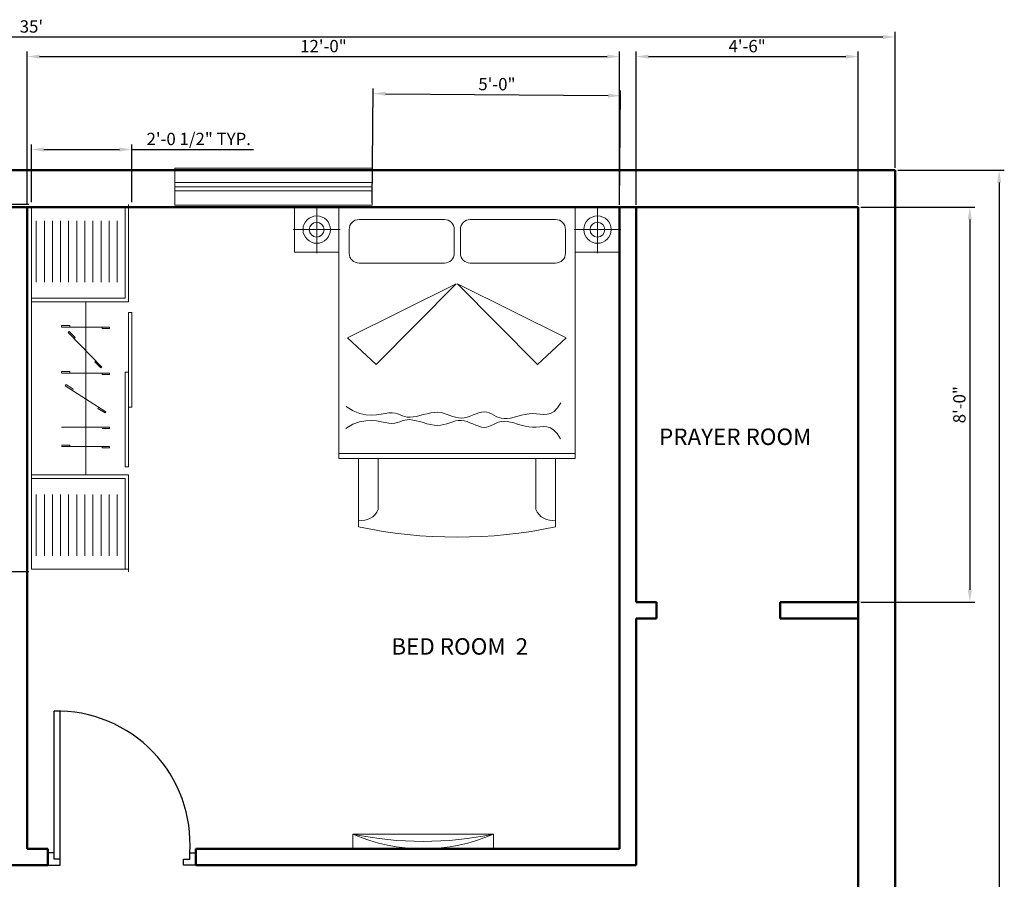
# Model space of a CAD drawing. Units: inches. Extents: x 108 to 1546, y -229 to 513.
# Tile 7 of 11: x 830 to 1070, y 304 to 513. Entities that reach past the tile are written whole.
import ezdxf

# ---------------------------------------------------------------- set-up
doc = ezdxf.new("R2010")
doc.units = ezdxf.units.IN
for name, color, linetype, lineweight in [('A-ANNO-DIMS', 2, 'Continuous', 18), ('A-AREA-IDEN', 4, 'Continuous', 18), ('A-FURN', 8, 'Continuous', 13), ('door', 1, 'Continuous', 25), ('tv', 2, 'Continuous', 13), ('wall', 7, 'Continuous', 50), ('WINDOW', 212, 'Continuous', 18)]:
    doc.layers.add(name, color=color, linetype=linetype, lineweight=lineweight)
doc.styles.get("Standard").update_dxf_attribs({"font": 'arial.ttf'})
doc.dimstyles.new('ISO-25', dxfattribs={"dimtxt": 3, "dimasz": 3, "dimexe": 1.25, "dimexo": 0.625, "dimtad": 1, "dimdec": 1, "dimlunit": 3, "dimtxsty": 'Standard', "dimcen": 2.5, "dimadec": 0, "dimazin": 0, "dimtfac": 1, "dimtdec": 1, "dimtmove": 0, "dimatfit": 3, "dimfxl": 1, "dimarcsym": 0})

# ---------------------------------------------------------------- blocks, each defined once
blk = doc.blocks.new('A$C4F543DC7')
for p, q in [((0.0134, 3.35, -0.1688), (3.3134, 3.35, -0.1688)), ((0.4634, 3.35, -0.1688), (0.0134, 3.35, -0.1688)), ((0.0134, 2.896, -0.1688), (0.0134, 3.35, -0.1688)), ((0.0134, 3.35, -0.1688), (0.0134, 2.896, -0.1688)), ((0.2381, 3.1233, -0.4388), (0.2381, 3.3614, -0.4388)), ((0.4634, 3.35, -0.1688), (0.4634, 0.8, -0.1688)), ((2.8634, 3.35, -0.1688), (0.4634, 3.35, -0.1688)), ((0.4634, 2.896, -0.1688), (0.4634, 3.35, -0.1688)), ((2.8634, 0.8, -0.1688), (2.8634, 3.35, -0.1688)), ((2.8634, 3.35, -0.1688), (3.3134, 3.35, -0.1688)), ((2.8634, 2.896, -0.1688), (2.8634, 3.35, -0.1688)), ((3.0888, 3.1233, -0.4388), (3.0888, 3.3614, -0.4388)), ((3.3134, 3.35, -0.1688), (3.3134, 2.896, -0.1688)), ((3.3134, 3.35, -0.1688), (3.3134, 2.896, -0.1688)), ((1.5354, 3.226, -0.1688), (0.6684, 3.226, -0.1688)), ((2.6644, 3.226, -0.1688), (1.7974, 3.226, -0.1688)), ((0.2381, 3.1233, -0.4388), (0, 3.1233, -0.4388)), ((0.2381, 3.1233, -0.4388), (0.4762, 3.1233, -0.4388)), ((0.2381, 3.1233, -0.4388), (0.2381, 2.8852, -0.4388)), ((0.5684, 3.126, -0.1688), (0.5684, 2.884, -0.1688)), ((1.6354, 2.884, -0.1688), (1.6354, 3.126, -0.1688)), ((1.6974, 3.126, -0.1688), (1.6974, 2.884, -0.1688)), ((2.7644, 2.884, -0.1688), (2.7644, 3.126, -0.1688)), ((3.0888, 3.1233, -0.4388), (2.8507, 3.1233, -0.4388)), ((3.0888, 3.1233, -0.4388), (3.0888, 2.8852, -0.4388)), ((3.0888, 3.1233, -0.4388), (3.3269, 3.1233, -0.4388)), ((0.4634, 2.896, -0.1688), (0.0134, 2.896, -0.1688)), ((0.0134, 2.896, -0.1688), (0.4634, 2.896, -0.1688)), ((0.4634, 0.8, -0.1688), (0.4634, 2.896, -0.1688)), ((2.8634, 2.896, -0.1688), (2.8634, 0.8, -0.1688)), ((3.3134, 2.896, -0.1688), (2.8634, 2.896, -0.1688)), ((3.3134, 2.896, -0.1688), (2.8634, 2.896, -0.1688)), ((0.6684, 2.784, -0.1688), (1.5354, 2.784, -0.1688)), ((1.7974, 2.784, -0.1688), (2.6644, 2.784, -0.1688)), ((1.6534, 2.573, -0.1688), (0.5504, 2.025, -0.1688)), ((0.8414, 1.752, -0.1688), (1.6534, 2.573, -0.1688)), ((2.4814, 1.752, -0.1688), (1.6694, 2.573, -0.1688)), ((1.6694, 2.573, -0.1688), (2.7724, 2.025, -0.1688)), ((0.5504, 2.025, -0.1688), (0.8414, 1.752, -0.1688)), ((2.7724, 2.025, -0.1688), (2.4814, 1.752, -0.1688)), ((0.5369, 1.3267, -0.1688), (0.6088, 1.2835, -0.1688)), ((2.6479, 1.2774, -0.1688), (2.683, 1.312, -0.1688)), ((2.683, 1.312, -0.1688), (2.7182, 1.3641, -0.1688)), ((0.6088, 1.2835, -0.1688), (0.6756, 1.2566, -0.1688)), ((0.6756, 1.2566, -0.1688), (0.7373, 1.2428, -0.1688)), ((0.7373, 1.2428, -0.1688), (0.794, 1.239, -0.1688)), ((0.794, 1.239, -0.1688), (0.8457, 1.242, -0.1688)), ((0.8457, 1.242, -0.1688), (0.8925, 1.2489, -0.1688)), ((0.8925, 1.2489, -0.1688), (0.9345, 1.2564, -0.1688)), ((0.9345, 1.2564, -0.1688), (0.9718, 1.2615, -0.1688)), ((0.9718, 1.2615, -0.1688), (1.0044, 1.2617, -0.1688)), ((1.0044, 1.2617, -0.1688), (1.0334, 1.2578, -0.1688)), ((1.0334, 1.2578, -0.1688), (1.0597, 1.2509, -0.1688)), ((1.0597, 1.2509, -0.1688), (1.0842, 1.2424, -0.1688)), ((1.0842, 1.2424, -0.1688), (1.1081, 1.2336, -0.1688)), ((1.1081, 1.2336, -0.1688), (1.1322, 1.2257, -0.1688)), ((1.1322, 1.2257, -0.1688), (1.1577, 1.2201, -0.1688)), ((1.1577, 1.2201, -0.1688), (1.1855, 1.218, -0.1688)), ((1.1855, 1.218, -0.1688), (1.2163, 1.2204, -0.1688)), ((1.2163, 1.2204, -0.1688), (1.2498, 1.2264, -0.1688)), ((1.2498, 1.2264, -0.1688), (1.2852, 1.2347, -0.1688)), ((1.2852, 1.2347, -0.1688), (1.3218, 1.2441, -0.1688)), ((1.3218, 1.2441, -0.1688), (1.3591, 1.2533, -0.1688)), ((1.3591, 1.2533, -0.1688), (1.3963, 1.2612, -0.1688)), ((1.3963, 1.2612, -0.1688), (1.4328, 1.2664, -0.1688)), ((1.4328, 1.2664, -0.1688), (1.4679, 1.2677, -0.1688)), ((1.4679, 1.2677, -0.1688), (1.501, 1.2643, -0.1688)), ((1.501, 1.2643, -0.1688), (1.5324, 1.257, -0.1688)), ((1.5324, 1.257, -0.1688), (1.5624, 1.2473, -0.1688)), ((1.5624, 1.2473, -0.1688), (1.5915, 1.2365, -0.1688)), ((1.5915, 1.2365, -0.1688), (1.6199, 1.2259, -0.1688)), ((1.6199, 1.2259, -0.1688), (1.6481, 1.2169, -0.1688)), ((1.6481, 1.2169, -0.1688), (1.6765, 1.2108, -0.1688)), ((1.6765, 1.2108, -0.1688), (1.7053, 1.209, -0.1688)), ((1.7053, 1.209, -0.1688), (1.7349, 1.2124, -0.1688)), ((1.7349, 1.2124, -0.1688), (1.7651, 1.2199, -0.1688)), ((1.7651, 1.2199, -0.1688), (1.7955, 1.2301, -0.1688)), ((1.7955, 1.2301, -0.1688), (1.8258, 1.2417, -0.1688)), ((1.8258, 1.2417, -0.1688), (1.8557, 1.2531, -0.1688)), ((1.8557, 1.2531, -0.1688), (1.8849, 1.263, -0.1688)), ((1.8849, 1.263, -0.1688), (1.913, 1.2698, -0.1688)), ((1.913, 1.2698, -0.1688), (1.9397, 1.2722, -0.1688)), ((1.9397, 1.2722, -0.1688), (1.9649, 1.2692, -0.1688)), ((1.9649, 1.2692, -0.1688), (1.989, 1.2617, -0.1688)), ((1.989, 1.2617, -0.1688), (2.0124, 1.2512, -0.1688)), ((2.0124, 1.2512, -0.1688), (2.0359, 1.2391, -0.1688)), ((2.0359, 1.2391, -0.1688), (2.0599, 1.2269, -0.1688)), ((2.0599, 1.2269, -0.1688), (2.0849, 1.216, -0.1688)), ((2.0849, 1.216, -0.1688), (2.1117, 1.2077, -0.1688)), ((2.1117, 1.2077, -0.1688), (2.1407, 1.2037, -0.1688)), ((2.1407, 1.2037, -0.1688), (2.1723, 1.2047, -0.1688)), ((2.1723, 1.2047, -0.1688), (2.2062, 1.21, -0.1688)), ((2.2062, 1.21, -0.1688), (2.242, 1.2182, -0.1688)), ((2.242, 1.2182, -0.1688), (2.2791, 1.2279, -0.1688)), ((2.2791, 1.2279, -0.1688), (2.3173, 1.2378, -0.1688)), ((2.3173, 1.2378, -0.1688), (2.3558, 1.2465, -0.1688)), ((2.3558, 1.2465, -0.1688), (2.3944, 1.2527, -0.1688)), ((2.3944, 1.2527, -0.1688), (2.4325, 1.255, -0.1688)), ((2.4325, 1.255, -0.1688), (2.4698, 1.2529, -0.1688)), ((2.4698, 1.2529, -0.1688), (2.5064, 1.2488, -0.1688)), ((2.5064, 1.2488, -0.1688), (2.5423, 1.2459, -0.1688)), ((2.5423, 1.2459, -0.1688), (2.5777, 1.2476, -0.1688)), ((2.5777, 1.2476, -0.1688), (2.6129, 1.257, -0.1688)), ((2.6129, 1.257, -0.1688), (2.6479, 1.2774, -0.1688)), ((0.5334, 1.105, -0.1688), (0.6067, 1.1458, -0.1688)), ((0.6067, 1.1458, -0.1688), (0.6743, 1.1706, -0.1688)), ((0.6743, 1.1706, -0.1688), (0.7364, 1.1825, -0.1688)), ((0.7364, 1.1825, -0.1688), (0.7931, 1.1846, -0.1688)), ((0.7931, 1.1846, -0.1688), (0.8447, 1.1799, -0.1688)), ((0.8447, 1.1799, -0.1688), (0.8913, 1.1716, -0.1688)), ((0.8913, 1.1716, -0.1688), (0.9331, 1.1628, -0.1688)), ((0.9331, 1.1628, -0.1688), (0.9701, 1.1565, -0.1688)), ((0.9701, 1.1565, -0.1688), (1.0027, 1.1552, -0.1688)), ((1.0027, 1.1552, -0.1688), (1.0318, 1.1582, -0.1688)), ((1.0318, 1.1582, -0.1688), (1.0583, 1.1642, -0.1688)), ((1.0583, 1.1642, -0.1688), (1.0831, 1.172, -0.1688)), ((1.0831, 1.172, -0.1688), (1.1072, 1.18, -0.1688)), ((1.1072, 1.18, -0.1688), (1.1316, 1.1872, -0.1688)), ((1.1316, 1.1872, -0.1688), (1.1573, 1.192, -0.1688)), ((1.1573, 1.192, -0.1688), (1.1851, 1.1932, -0.1688)), ((1.1851, 1.1932, -0.1688), (1.2158, 1.1898, -0.1688)), ((1.2158, 1.1898, -0.1688), (1.2491, 1.1828, -0.1688)), ((1.2491, 1.1828, -0.1688), (1.2842, 1.1734, -0.1688)), ((1.2842, 1.1734, -0.1688), (1.3206, 1.1629, -0.1688)), ((1.3206, 1.1629, -0.1688), (1.3575, 1.1524, -0.1688)), ((1.3575, 1.1524, -0.1688), (1.3945, 1.1434, -0.1688)), ((1.3945, 1.1434, -0.1688), (1.4308, 1.1371, -0.1688)), ((1.4308, 1.1371, -0.1688), (1.4658, 1.1347, -0.1688)), ((1.4658, 1.1347, -0.1688), (1.499, 1.137, -0.1688)), ((1.499, 1.137, -0.1688), (1.5306, 1.1433, -0.1688)), ((1.5306, 1.1433, -0.1688), (1.5609, 1.152, -0.1688)), ((1.5609, 1.152, -0.1688), (1.5903, 1.1619, -0.1688)), ((1.5903, 1.1619, -0.1688), (1.6191, 1.1716, -0.1688)), ((1.6191, 1.1716, -0.1688), (1.6475, 1.1797, -0.1688)), ((1.6475, 1.1797, -0.1688), (1.676, 1.1849, -0.1688)), ((1.676, 1.1849, -0.1688), (1.7049, 1.1858, -0.1688)), ((1.7049, 1.1858, -0.1688), (1.7344, 1.1816, -0.1688)), ((1.7344, 1.1816, -0.1688), (1.7643, 1.1731, -0.1688)), ((1.7643, 1.1731, -0.1688), (1.7944, 1.1619, -0.1688)), ((1.7944, 1.1619, -0.1688), (1.8244, 1.1494, -0.1688)), ((1.8244, 1.1494, -0.1688), (1.8539, 1.137, -0.1688)), ((1.8539, 1.137, -0.1688), (1.8827, 1.1263, -0.1688)), ((1.8827, 1.1263, -0.1688), (1.9106, 1.1186, -0.1688)), ((1.9106, 1.1186, -0.1688), (1.9373, 1.1153, -0.1688)), ((1.9373, 1.1153, -0.1688), (1.9625, 1.1176, -0.1688)), ((1.9625, 1.1176, -0.1688), (1.9868, 1.1243, -0.1688)), ((1.9868, 1.1243, -0.1688), (2.0106, 1.134, -0.1688)), ((2.0106, 1.134, -0.1688), (2.0344, 1.1454, -0.1688)), ((2.0344, 1.1454, -0.1688), (2.0588, 1.1568, -0.1688)), ((2.0588, 1.1568, -0.1688), (2.0842, 1.167, -0.1688)), ((2.0842, 1.167, -0.1688), (2.1112, 1.1743, -0.1688)), ((2.1112, 1.1743, -0.1688), (2.1403, 1.1775, -0.1688)), ((2.1403, 1.1775, -0.1688), (2.1718, 1.1755, -0.1688)), ((2.1718, 1.1755, -0.1688), (2.2056, 1.1691, -0.1688)), ((2.2056, 1.1691, -0.1688), (2.2411, 1.1598, -0.1688)), ((2.2411, 1.1598, -0.1688), (2.2779, 1.1489, -0.1688)), ((2.2779, 1.1489, -0.1688), (2.3157, 1.1379, -0.1688)), ((2.3157, 1.1379, -0.1688), (2.354, 1.1279, -0.1688)), ((2.354, 1.1279, -0.1688), (2.3923, 1.1205, -0.1688)), ((2.3923, 1.1205, -0.1688), (2.4304, 1.117, -0.1688)), ((2.4304, 1.117, -0.1688), (2.4677, 1.118, -0.1688)), ((2.4677, 1.118, -0.1688), (2.5043, 1.1209, -0.1688)), ((2.5043, 1.1209, -0.1688), (2.5403, 1.1226, -0.1688)), ((2.5403, 1.1226, -0.1688), (2.5757, 1.1199, -0.1688)), ((2.5757, 1.1199, -0.1688), (2.6106, 1.1094, -0.1688)), ((2.6106, 1.1094, -0.1688), (2.645, 1.0879, -0.1688)), ((2.645, 1.0879, -0.1688), (2.6789, 1.0522, -0.1688)), ((2.6789, 1.0522, -0.1688), (2.7124, 0.999, -0.1688)), ((0.4634, 0.85, -0.1688), (2.8634, 0.85, -0.1688)), ((0.4634, 0.8, -0.1688), (2.8634, 0.8, -0.1688)), ((0.6634, 0.8, -0.1688), (0.4634, 0.8, -0.1688)), ((0.6634, 0.8, -0.1688), (2.6634, 0.8, -0.1688)), ((0.6634, 0.104, -0.1688), (0.6634, 0.8, -0.1688)), ((0.6634, 0.104, -0.1688), (0.6634, 0.8, -0.1688)), ((0.8634, 0.281, -0.1688), (0.8634, 0.8, -0.1688)), ((2.4634, 0.8, -0.1688), (2.4634, 0.281, -0.1688)), ((2.8634, 0.8, -0.1688), (2.6634, 0.8, -0.1688)), ((2.6634, 0.8, -0.1688), (2.6634, 0.104, -0.1688)), ((2.6634, 0.8, -0.1688), (2.6634, 0.104, -0.1688))]:
    blk.add_line(p, q)
for centre, radius in [((0.2381, 3.1233, -0.4388), 0.139), ((3.0888, 3.1233, -0.4388), 0.139), ((0.2381, 3.1233, -0.4388), 0.075), ((3.0888, 3.1233, -0.4388), 0.075)]:
    blk.add_circle(centre, radius)
for centre, radius, start, end in [((0.6684, 3.126, -0.1688), 0.1, 90, 180), ((1.5354, 3.126, -0.1688), 0.1, 0, 90), ((1.7974, 3.126, -0.1688), 0.1, 90, 180), ((2.6644, 3.126, -0.1688), 0.1, 0, 90), ((0.6684, 2.884, -0.1688), 0.1, 180, 270), ((1.5354, 2.884, -0.1688), 0.1, 270, 0), ((1.7974, 2.884, -0.1688), 0.1, 180, 270), ((2.6644, 2.884, -0.1688), 0.1, 270, 0), ((0.6994, 0.3472, -0.1688), 0.1769, 258.2616, 338.03196), ((2.6275, 0.3472, -0.1688), 0.1769, 201.96804, 281.7384), ((1.6634, 4.8597, -0.1688), 4.8597, 258.12517, 281.87483), ((1.6634, 4.8597, -0.1688), 4.8597, 258.12517, 281.87483)]:
    blk.add_arc(centre, radius, start, end)
blk = doc.blocks.new('A$C34930FF8')
at = {"ltscale": 0.05}
for p, q in [((0, 2252.4), (0, 16.8)), ((600, 2252.4), (0, 2252.4)), ((185.4, 1513), (185.4, 1521.5)), ((237.7, 1513), (237.7, 1521.5)), ((227.1, 1479.2), (233.2, 1485.2)), ((436.7, 1513), (436.7, 1504.4)), ((482.5, 1513), (482.5, 1504.4)), ((263.6, 1441.7), (269.7, 1447.7)), ((398.2, 1303.6), (392.1, 1297.6)), ((185.4, 1229.1), (185.4, 1237.7)), ((237.7, 1229.1), (237.7, 1237.7)), ((434.8, 1266.1), (428.7, 1260.1)), ((436.7, 1228.2), (436.7, 1219.7)), ((482.5, 1228.2), (482.5, 1219.7)), ((209.5, 1150.1), (214.1, 1157.3)), ((253.5, 1121.8), (258.1, 1129)), ((415.3, 1017.6), (410.6, 1010.5)), ((459.3, 989.3), (454.7, 982.1)), ((482.5, 894.9), (482.5, 886.3)), ((237.7, 775.3), (237.7, 783.9)), ((436.7, 775.3), (436.7, 766.8)), ((482.5, 775.3), (482.5, 766.8)), ((600, 16.8), (0, 16.8))]:
    blk.add_line(p, q, dxfattribs=at)
for p, q in [((580, 1690.9), (580, 2252.4)), ((600, 1669.3), (600, 2269.3)), ((30, 1790.9), (30, 2169.3)), ((80, 1790.9), (80, 2169.3)), ((130, 1790.9), (130, 2169.3)), ((180, 1790.9), (180, 2169.3)), ((230, 1790.9), (230, 2169.3)), ((280, 1790.9), (280, 2169.3)), ((330, 1790.9), (330, 2169.3)), ((380, 1790.9), (380, 2169.3)), ((430, 1790.9), (430, 2169.3)), ((480, 1790.9), (480, 2169.3)), ((530, 1790.9), (530, 2169.3)), ((580, 1690.9), (0, 1690.9)), ((600, 1669.3), (0, 1669.3)), ((335.4, 1666.1), (335.4, 603.1)), ((600, 1603.3), (620, 1603.3)), ((600, 1018.7), (600, 1603.3)), ((620, 1603.3), (620, 1018.7)), ((237.7, 1521.5), (185.4, 1521.5)), ((482.5, 1513), (185.4, 1513)), ((434.8, 1266.1), (227.4, 1478.9)), ((269.7, 1447.7), (233.2, 1485.2)), ((436.7, 1504.4), (482.5, 1504.4)), ((428.7, 1260.1), (392.1, 1297.6)), ((237.7, 1237.7), (185.4, 1237.7)), ((482.5, 1228.2), (185.4, 1228.2)), ((436.7, 1219.7), (482.5, 1219.7)), ((600, 1233.4), (580, 1233.4)), ((580, 1233.4), (580, 648.7)), ((600, 648.7), (600, 1233.4)), ((258.1, 1129), (214.1, 1157.3)), ((459.3, 989.3), (209.5, 1150.1)), ((454.7, 982.1), (410.6, 1010.5)), ((620, 1018.7), (600, 1018.7)), ((482.5, 894.9), (185.4, 894.9)), ((436.7, 886.3), (482.5, 886.3)), ((237.7, 783.9), (185.4, 783.9)), ((482.5, 775.3), (185.4, 775.3)), ((436.7, 766.8), (482.5, 766.8)), ((580, 648.7), (600, 648.7)), ((600, 600), (0, 600)), ((580, 578.3), (0, 578.3)), ((580, 578.3), (580, 16.8)), ((600, 600), (600, 0)), ((30, 478.3), (30, 100)), ((80, 478.3), (80, 100)), ((130, 478.3), (130, 100)), ((180, 478.3), (180, 100)), ((230, 478.3), (230, 100)), ((280, 478.3), (280, 100)), ((330, 478.3), (330, 100)), ((380, 478.3), (380, 100)), ((430, 478.3), (430, 100)), ((480, 478.3), (480, 100)), ((530, 478.3), (530, 100))]:
    blk.add_line(p, q)
blk = doc.blocks.new('*D23')
at = {"layer": 'A-ANNO-DIMS', "color": 0, "lineweight": -2, "transparency": 16777216}
for p, q in [((623, 477.09), (623, 510.15)), ((1043, 477.09), (1043, 510.15)), ((626, 508.9), (1040, 508.9))]:
    blk.add_line(p, q, dxfattribs=at)
at = {"layer": 'A-ANNO-DIMS', "color": 0, "transparency": 16777216}
for points in [[(626, 509.4), (626, 508.4), (623, 508.9)], [(1040, 509.4), (1040, 508.4), (1043, 508.9)]]:
    blk.add_solid(points, dxfattribs=at)
at = {"layer": 'Defpoints', "color": 0, "transparency": 16777216}
for p in [(1043, 508.9), (623, 476.47), (1043, 476.47)]:
    blk.add_point(p, dxfattribs=at)
at = {"layer": 'A-ANNO-DIMS', "color": 0, "transparency": 16777216, "insert": (833, 511.06), "char_height": 3, "attachment_point": 5}
blk.add_mtext("35'", dxfattribs=at)
blk = doc.blocks.new('*D24')
at = {"layer": 'A-ANNO-DIMS', "color": 0, "lineweight": -2, "transparency": 16777216}
for p, q in [((1043.62, 476.47), (1069.53, 476.47)), ((1068.28, 473.47), (1068.28, -0.53)), ((1043.62, -3.53), (1069.53, -3.53))]:
    blk.add_line(p, q, dxfattribs=at)
at = {"layer": 'A-ANNO-DIMS', "color": 0, "transparency": 16777216}
for points in [[(1067.78, 473.47), (1068.78, 473.47), (1068.28, 476.47)], [(1067.78, -0.53), (1068.78, -0.53), (1068.28, -3.53)]]:
    blk.add_solid(points, dxfattribs=at)
at = {"layer": 'Defpoints', "color": 0, "transparency": 16777216}
for p in [(1043, 476.47), (1043, -3.53), (1068.28, -3.53)]:
    blk.add_point(p, dxfattribs=at)
at = {"layer": 'A-ANNO-DIMS', "color": 0, "transparency": 16777216, "insert": (1066.12, 236.47), "char_height": 3, "attachment_point": 5, "rotation": 90}
blk.add_mtext("40'", dxfattribs=at)
blk = doc.blocks.new('WINDOW-48X9')
for p, q in [((0, 9), (0, 0)), ((0, 9), (48, 9)), ((48, 9), (48, 0)), ((0, 5.5), (48, 5.5)), ((0, 4.5), (48, 4.5)), ((0, 3.5), (48, 3.5)), ((0, 0), (48, 0))]:
    blk.add_line(p, q)
blk = doc.blocks.new('DOOR-SWING-36')
for p, q in [((1.5, 1.5), (1.5, 37.5)), ((3, 1.5), (3, 37.5)), ((0, 3), (0, 0)), ((1.5, 3), (0, 3)), ((1.5, 1.5), (1.5, 3)), ((34.5, 1.5), (34.5, 3)), ((34.5, 3), (36, 3)), ((36, 3), (36, 0)), ((3, 1.5), (1.5, 1.5)), ((3, 0), (3, 1.5)), ((33, 0), (33, 1.5)), ((33, 1.5), (34.5, 1.5)), ((0, 0), (3, 0)), ((36, 0), (33, 0))]:
    blk.add_line(p, q)
blk.add_arc((2.25, 5.18), 32.32, 356.1244, 91.3295)
blk = doc.blocks.new('TV-WALL-MOUNT')
blk.add_lwpolyline([(0, 0), (34.19, 0), (34.19, 3.56), (0, 3.56)], close=True)
for centre, radius, start, end in [((17.1, 42.8), 42.8, 246.4582, 293.5418), ((17.1, 84.72), 82.93, 258.1036, 281.8964)]:
    blk.add_arc(centre, radius, start, end)
blk = doc.blocks.new('*D44')
at = {"layer": 'A-ANNO-DIMS', "color": 0, "lineweight": -2, "transparency": 16777216}
for p, q in [((832.37, 468.13), (818.34, 468.13)), ((819.59, 381.79), (819.59, 465.13)), ((832.37, 378.79), (818.34, 378.79))]:
    blk.add_line(p, q, dxfattribs=at)
at = {"layer": 'A-ANNO-DIMS', "color": 0, "transparency": 16777216}
for points in [[(819.09, 465.13), (820.09, 465.13), (819.59, 468.13)], [(819.09, 381.79), (820.09, 381.79), (819.59, 378.79)]]:
    blk.add_solid(points, dxfattribs=at)
at = {"layer": 'Defpoints', "color": 0, "transparency": 16777216}
for p in [(819.59, 468.13), (833, 468.13), (833, 378.79)]:
    blk.add_point(p, dxfattribs=at)
at = {"layer": 'A-ANNO-DIMS', "color": 0, "transparency": 16777216, "insert": (817.42, 423.46), "char_height": 3, "attachment_point": 5, "rotation": 90}
blk.add_mtext('ROBE 7\'-5 1/2" TYP.', dxfattribs=at)
blk = doc.blocks.new('*D45')
at = {"layer": 'A-ANNO-DIMS', "color": 0, "lineweight": -2, "transparency": 16777216}
for p, q in [((833, 468.76), (833, 482.78)), ((836, 481.53), (854.4, 481.53)), ((857.4, 468.76), (857.4, 482.78)), ((857.4, 481.53), (886.98, 481.53))]:
    blk.add_line(p, q, dxfattribs=at)
at = {"layer": 'A-ANNO-DIMS', "color": 0, "transparency": 16777216}
for points in [[(836, 482.03), (836, 481.03), (833, 481.53)], [(854.4, 482.03), (854.4, 481.03), (857.4, 481.53)]]:
    blk.add_solid(points, dxfattribs=at)
at = {"layer": 'Defpoints', "color": 0, "transparency": 16777216}
for p in [(857.4, 481.53), (833, 468.13), (857.4, 468.13)]:
    blk.add_point(p, dxfattribs=at)
at = {"layer": 'A-ANNO-DIMS', "color": 0, "transparency": 16777216, "insert": (873.69, 483.71), "char_height": 3, "attachment_point": 5}
blk.add_mtext('2\'-0 1/2" TYP.', dxfattribs=at)
blk = doc.blocks.new('*D85')
at = {"layer": 'A-ANNO-DIMS', "color": 0, "lineweight": -2, "transparency": 16777216}
for p, q in [((832, 468.09), (832, 505.38)), ((976, 468.09), (976, 505.38)), ((835, 504.13), (973, 504.13))]:
    blk.add_line(p, q, dxfattribs=at)
at = {"layer": 'A-ANNO-DIMS', "color": 0, "transparency": 16777216}
for points in [[(835, 504.63), (835, 503.63), (832, 504.13)], [(973, 504.63), (973, 503.63), (976, 504.13)]]:
    blk.add_solid(points, dxfattribs=at)
at = {"layer": 'Defpoints', "color": 0, "transparency": 16777216}
for p in [(976, 504.13), (832, 467.47), (976, 467.47)]:
    blk.add_point(p, dxfattribs=at)
at = {"layer": 'A-ANNO-DIMS', "color": 0, "transparency": 16777216, "insert": (904, 506.28), "char_height": 3, "attachment_point": 5}
blk.add_mtext('12\'-0"', dxfattribs=at)
blk = doc.blocks.new('*D86')
at = {"layer": 'A-ANNO-DIMS', "color": 0, "lineweight": -2, "transparency": 16777216}
for p, q in [((980, 468.09), (980, 505.38)), ((1034, 468.09), (1034, 505.38)), ((983, 504.13), (1031, 504.13))]:
    blk.add_line(p, q, dxfattribs=at)
at = {"layer": 'A-ANNO-DIMS', "color": 0, "transparency": 16777216}
for points in [[(983, 504.63), (983, 503.63), (980, 504.13)], [(1031, 504.63), (1031, 503.63), (1034, 504.13)]]:
    blk.add_solid(points, dxfattribs=at)
at = {"layer": 'Defpoints', "color": 0, "transparency": 16777216}
for p in [(1034, 504.13), (980, 467.47), (1034, 467.47)]:
    blk.add_point(p, dxfattribs=at)
at = {"layer": 'A-ANNO-DIMS', "color": 0, "transparency": 16777216, "insert": (1007, 506.28), "char_height": 3, "attachment_point": 5}
blk.add_mtext('4\'-6"', dxfattribs=at)
blk = doc.blocks.new('*D97')
at = {"layer": 'A-ANNO-DIMS', "color": 0, "lineweight": -2, "transparency": 16777216}
for p, q in [((1034.62, 467.47), (1062.4, 467.47)), ((1061.15, 464.47), (1061.15, 374.47)), ((1034.62, 371.47), (1062.4, 371.47))]:
    blk.add_line(p, q, dxfattribs=at)
at = {"layer": 'A-ANNO-DIMS', "color": 0, "transparency": 16777216}
for points in [[(1060.65, 464.47), (1061.65, 464.47), (1061.15, 467.47)], [(1060.65, 374.47), (1061.65, 374.47), (1061.15, 371.47)]]:
    blk.add_solid(points, dxfattribs=at)
at = {"layer": 'Defpoints', "color": 0, "transparency": 16777216}
for p in [(1034, 467.47), (1034, 371.47), (1061.15, 371.47)]:
    blk.add_point(p, dxfattribs=at)
at = {"layer": 'A-ANNO-DIMS', "color": 0, "transparency": 16777216, "insert": (1058.99, 419.47), "char_height": 3, "attachment_point": 5, "rotation": 90}
blk.add_mtext('8\'-0"', dxfattribs=at)
blk = doc.blocks.new('*D100')
at = {"layer": 'A-ANNO-DIMS', "color": 0, "lineweight": -2, "transparency": 16777216}
for p, q in [((915.86, 468.6), (916.09, 496.38)), ((976, 468.09), (976.24, 495.87)), ((919.08, 495.1), (973.22, 494.64))]:
    blk.add_line(p, q, dxfattribs=at)
at = {"layer": 'A-ANNO-DIMS', "color": 0, "transparency": 16777216}
for points in [[(919.09, 495.6), (919.08, 494.6), (916.08, 495.13)], [(973.23, 495.14), (973.22, 494.14), (976.22, 494.62)]]:
    blk.add_solid(points, dxfattribs=at)
at = {"layer": 'Defpoints', "color": 0, "transparency": 16777216}
for p in [(976.22, 494.62), (915.85, 467.98), (976, 467.47)]:
    blk.add_point(p, dxfattribs=at)
at = {"layer": 'A-ANNO-DIMS', "color": 0, "transparency": 16777216, "insert": (946.17, 497.03), "char_height": 3, "attachment_point": 5, "rotation": 359.5159}
blk.add_mtext('5\'-0"', dxfattribs=at)

msp = doc.modelspace()

# ---------------------------------------------------------------- linework, layer by layer
at = {"layer": 'wall'}
for p, q in [((1043, 476.47), (623, 476.47)), ((1043, -3.53), (1043, 476.47)), ((1034, 467.47), (632, 467.47)), ((832, 467.47), (832, 311.47)), ((976, 467.47), (976, 311.47)), ((980, 467.47), (980, 371.47)), ((1034, 5.47), (1034, 467.47)), ((985, 371.47), (980, 371.47)), ((985, 371.47), (985, 367.47)), ((1034, 371.47), (1015, 371.47)), ((1015, 371.47), (1015, 367.47)), ((980, 367.47), (980, 307.47)), ((985, 367.47), (980, 367.47)), ((1034, 367.47), (1015, 367.47)), ((837, 311.47), (832, 311.47)), ((837, 311.47), (837, 307.47)), ((976, 311.47), (873, 311.47)), ((873, 311.47), (873, 307.47)), ((976, 311.47), (914, 311.47)), ((837, 307.47), (821, 307.47)), ((980, 307.47), (873, 307.47)), ((980, 307.47), (914, 307.47))]:
    msp.add_line(p, q, dxfattribs=at)

# ---------------------------------------------------------------- block references
at = {"layer": 'A-FURN'}
for name, p, xscale, yscale, zscale in [('A$C34930FF8', (833, 378.79), 0.0393700787401575, 0.0393700787401575, 0.0393700787401575), ('A$C4F543DC7', (896.66, 387.26, 4.04), 23.94379789781286, 23.94379789781286, 23.94379789781286)]:
    msp.add_blockref(name, p, dxfattribs=dict(at, xscale=xscale, yscale=yscale, zscale=zscale))
at = {"layer": 'door'}
msp.add_blockref('DOOR-SWING-36', (837, 307.47), dxfattribs=at)
at = {"layer": 'tv'}
msp.add_blockref('TV-WALL-MOUNT', (911.14, 311.47), dxfattribs=at)
at = {"layer": 'WINDOW', "rotation": 180}
msp.add_blockref('WINDOW-48X9', (915.85, 476.98), dxfattribs=at)

# ---------------------------------------------------------------- texts
at = {"layer": 'A-AREA-IDEN', "char_height": 4, "attachment_point": 1}
for s, insert in [('PRAYER ROOM', (985.59, 413.67)), ('BED ROOM  2', (920.52, 362.69))]:
    msp.add_mtext_dynamic_manual_height_columns(s, width=57.4311, gutter_width=12.5, heights=[12.84], dxfattribs=dict(at, insert=insert))

# ---------------------------------------------------------------- dimensions: what is measured, and where the dimension line sits
at = {"layer": 'A-ANNO-DIMS'}
for base, p1, p2, override, picture, middle in [((1043, 508.9), (623, 476.47), (1043, 476.47), {"dimclrd": 0, "dimclre": 0, "dimclrt": 0}, '*D23', (833, 511.06)), ((976, 504.13), (832, 467.47), (976, 467.47), {"dimdec": 1, "dimlfac": 1, "dimrnd": 0, "dimzin": 1, "dimdsep": 46, "dimlunit": 4, "dimfrac": 2}, '*D85', (904, 506.28)), ((1034, 504.13), (980, 467.47), (1034, 467.47), {"dimdec": 1, "dimlfac": 1, "dimrnd": 0, "dimzin": 1, "dimdsep": 46, "dimlunit": 4, "dimfrac": 2}, '*D86', (1007, 506.28))]:
    dim = msp.add_linear_dim(base=base, p1=p1, p2=p2, dimstyle='ISO-25', override=override, dxfattribs=at)
    dim.commit()
    dim.dimension.update_dxf_attribs({"geometry": picture, "text_midpoint": middle})
for base, p1, p2, angle, override, picture, middle in [((976.2245, 494.6189), (915.8535, 467.9781), (975.9951, 467.4699), 359.5159, {"dimdec": 1, "dimlfac": 1, "dimrnd": 0, "dimzin": 1, "dimdsep": 46, "dimlunit": 4, "dimfrac": 2}, '*D100', (946.1719, 497.0297)), ((1068.28, -3.53), (1043, 476.47), (1043, -3.53), 90, {"dimclrd": 0, "dimclre": 0, "dimclrt": 0}, '*D24', (1066.12, 236.47)), ((1061.15, 371.47), (1034, 467.47), (1034, 371.47), 270, {"dimdec": 1, "dimlfac": 1, "dimrnd": 0, "dimzin": 1, "dimdsep": 46, "dimlunit": 4, "dimfrac": 2}, '*D97', (1058.99, 419.47))]:
    dim = msp.add_linear_dim(base=base, p1=p1, p2=p2, angle=angle, dimstyle='ISO-25', override=override, dxfattribs=at)
    dim.commit()
    dim.dimension.update_dxf_attribs({"geometry": picture, "text_midpoint": middle})
dim = msp.add_linear_dim(base=(857.4, 481.53), p1=(833, 468.13), p2=(857.4, 468.13), text='<> TYP.', dimstyle='ISO-25', override={"dimdec": 1, "dimlfac": 1, "dimrnd": 0, "dimzin": 1, "dimdsep": 46, "dimlunit": 4, "dimfrac": 2}, dxfattribs=at)
dim.commit()
dim.dimension.update_dxf_attribs({"geometry": '*D45', "text_midpoint": (873.69, 483.71)})
dim = msp.add_linear_dim(base=(819.59, 468.13), p1=(833, 378.79), p2=(833, 468.13), angle=90, text='ROBE <> TYP.', dimstyle='ISO-25', override={"dimdec": 1, "dimlfac": 1, "dimrnd": 0, "dimzin": 1, "dimdsep": 46, "dimlunit": 4, "dimfrac": 2}, dxfattribs=at)
dim.commit()
dim.dimension.update_dxf_attribs({"geometry": '*D44', "text_midpoint": (817.42, 423.46)})

doc.saveas('drawing.dxf')
